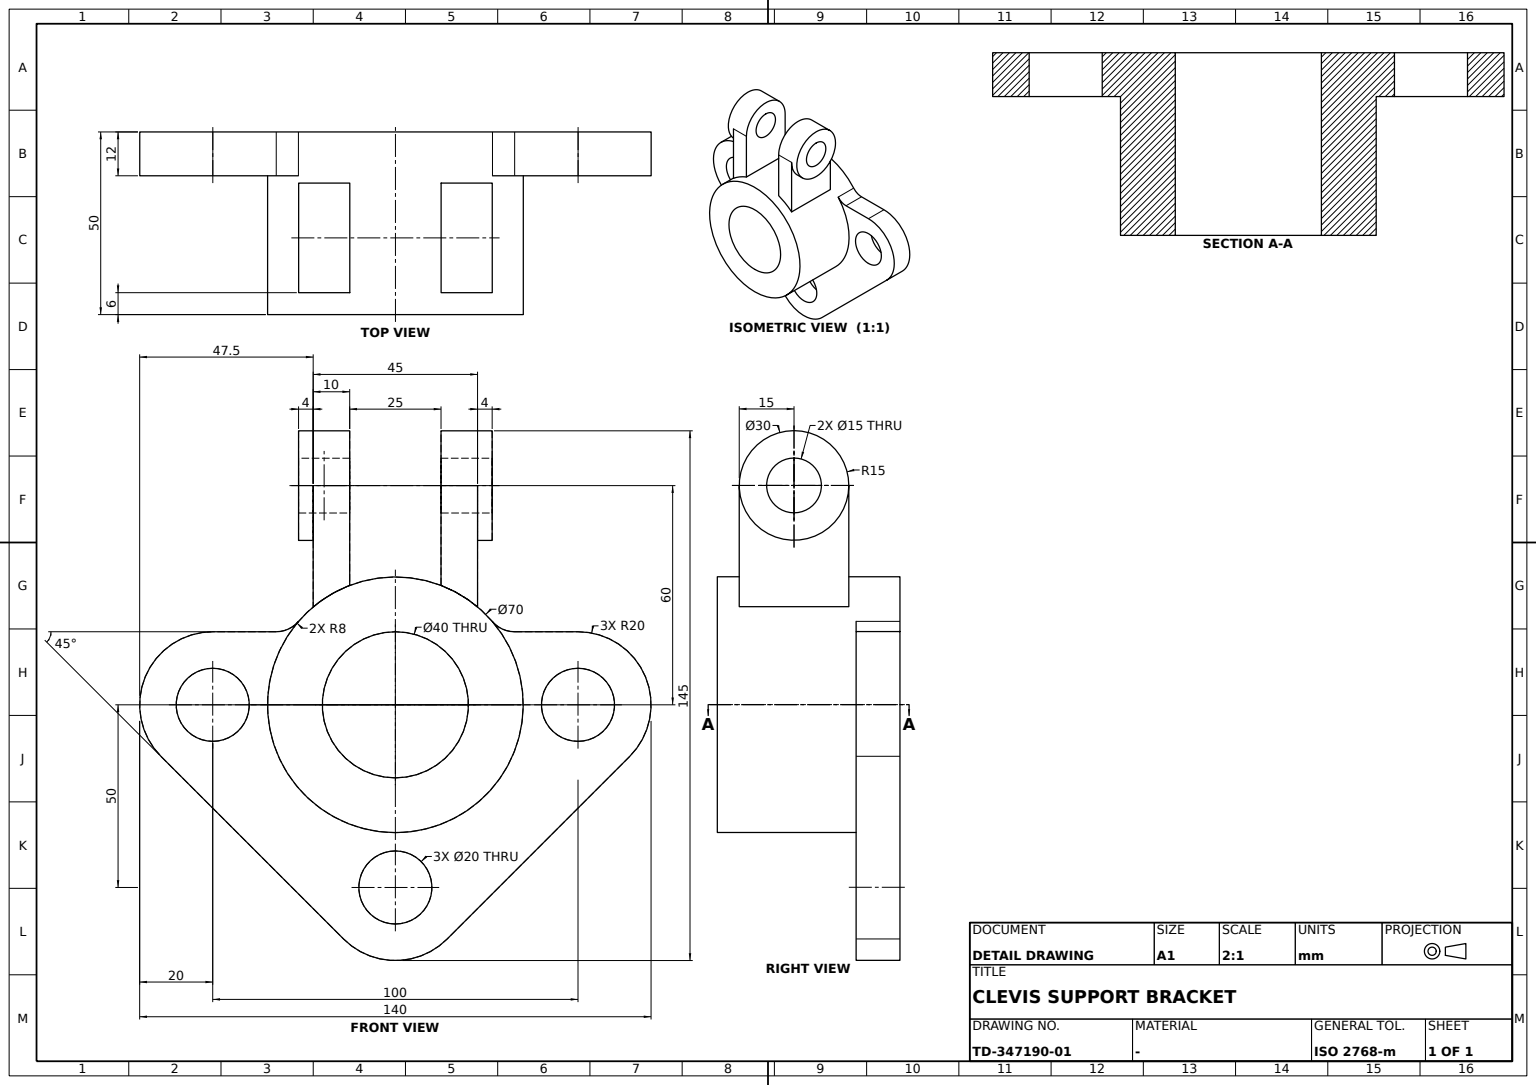
CATIA V5 part; units mm, degrees
sketch "Sketch1" plane through (0, 0, 0) normal (1, 0, 0) x (0, 1, 0)
  circle A0 centre (0, 0) radius 35
  circle A1 centre (0, 0) radius 20
  dimension "radius A1" = 20
  dimension "radius A0" = 35
extrude "Pad1" add sketch "Sketch1" along normal blind 50
sketch "Sketch2" plane through (0, 0, 0) normal (1, 0, 0) x (0, 1, 0)
  circle A0 centre (0, 0) radius 35 construction
  arc A1 (26.5628, 22.7907) -> (-26.5628, 22.7907) centre (0, 0) ccw
  circle A2 centre (50, 0) radius 10
  point P0 (50, 0)
  circle A3 centre (0, -50) radius 10
  point P1 (0, -50)
  line L0 (0, -50) -> (29.5938, -50) construction
  circle A4 centre (-50, 0) radius 10
  arc A5 (-50, 20) -> (-64.1421, -14.1421) centre (-50, 0) ccw
  arc A6 (-14.1421, -64.1421) -> (14.1421, -64.1421) centre (0, -50) ccw
  arc A7 (64.1421, -14.1421) -> (50, 20) centre (50, 0) ccw
  line L1 (-50, 20) -> (-32.6343, 20)
  line L2 (-64.1421, -14.1421) -> (-14.1421, -64.1421)
  line L3 (14.1421, -64.1421) -> (64.1421, -14.1421)
  point P2 (28.7228, 20)
  line L4 (32.6343, 20) -> (50, 20)
  point P3 (28.7228, 20)
  arc A8 (-26.5628, 22.7907) -> (-32.6343, 20) centre (-32.6343, 28) cw
  arc A9 (26.5628, 22.7907) -> (32.6343, 20) centre (32.6343, 28) ccw
  circle A10 centre (0, 0) radius 20
  dimension "radius A2" = 10
  dimension "distance y axis P0" = 50
  dimension "radius A3" = 10
  dimension "distance P1 x axis" = 50
  dimension "distance L0 P0" = 50
  dimension "radius A7" = 20
  dimension "radius A6" = 20
  dimension "radius A5" = 20
  dimension "radius A8" = 8
  dimension "radius A9" = 8
  constraint coincidence P1 y-axis
  constraint coincidence L1 P2
  constraint coincidence A0 P3
  constraint coincidence L1 L4
  constraint coincidence A0 P2
  constraint coincidence L4 P3
  constraint horizontal L0 x-axis
  constraint symmetry A2 A4 y-axis
  constraint tangency L1 A7
  constraint tangency A5 L1
  constraint tangency L2 A5
  constraint tangency L2 A6
  constraint tangency L3 A7
  constraint tangency L3 A6
  constraint tangency A8 L1
  constraint tangency A8 A0
  constraint tangency A9 A0
  constraint tangency A9 L4
extrude "Pad2" add sketch "Sketch2" along normal blind 12
sketch "Sketch3" plane through (0, 0, 0) normal (0, 1, 0) x (-1, 0, 0)
  arc A0 (-14, 60) -> (-44, 60) centre (-29, 60) ccw
  point P0 (-29, 60)
  line L0 (-44, 60) -> (-14, 60) construction
  line L1 (-14, 60) -> (-14, 25)
  line L2 (-14, 25) -> (-44, 25)
  line L3 (-44, 25) -> (-44, 60)
  line L4 (-50, -35) -> (-50, 35) construction
  circle A1 centre (-29, 60) radius 7.5
  dimension "radius A0" = 15
  dimension "distance A0 x axis" = 45
  dimension "distance L4 L3" = 6
  dimension "distance L2 P0" = 35
  dimension "radius A1" = 7.5
  constraint horizontal L0 x-axis
  constraint horizontal L2 x-axis
  constraint tangency L1 A0
  constraint tangency L3 A0
extrude "Pad3" add sketch "Sketch3" along normal mid plane 45
sketch "Sketch4" plane through (0, 0, 0) normal (1, 0, 0) x (0, 1, 0)
  line L0 (-12.5, 91.649) -> (12.5, 91.649)
  line L1 (12.5, 91.649) -> (12.5, 32.6917)
  line L2 (-12.5, 32.6917) -> (-12.5, 91.649)
  circle A0 centre (0, 0) radius 35 construction
  arc A1 (12.5, 32.6917) -> (-12.5, 32.6917) centre (0, 0) ccw
  point P0 (-12.5, 32.6917)
  point P1 (12.5, 32.6917)
  point P2 (-12.5, 32.6917)
  point P3 (12.5, 32.6917)
  dimension "length L0" = 25
  constraint horizontal L0 x-axis
  constraint vertical L1 y-axis
  constraint vertical L2 y-axis
  constraint symmetry L2 L1 y-axis
  constraint coincidence L2 P0
  constraint coincidence L1 P1
  constraint coincidence A0 P2
  constraint coincidence A0 P3
  constraint coincidence P0 P2
  constraint coincidence P1 P3
extrude "Pocket1" cut sketch "Sketch4" along normal blind 50
sketch "Sketch5" plane through (0, 22.5, 0) normal (0, 1, 0) x (-1, 0, 0)
  circle A0 centre (-29, 60) radius 15
  arc A1 (-14, 60) -> (-44, 60) centre (-29, 60) ccw construction
  circle A2 centre (-29, 60) radius 7.5
  dimension "radius A0" = 15
  constraint concentricity A0 A1
extrude "Pad4" add sketch "Sketch5" along normal blind 4
mirror "Mirror1" about plane through (0, 0, 0) normal (0, 1, 0) of "Pad4"
properties part number "19"
